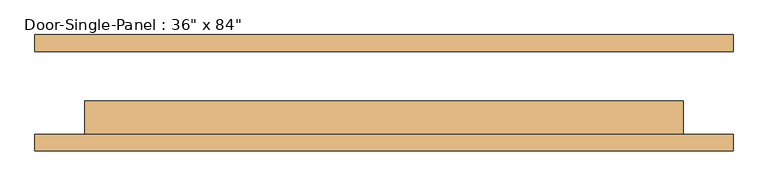
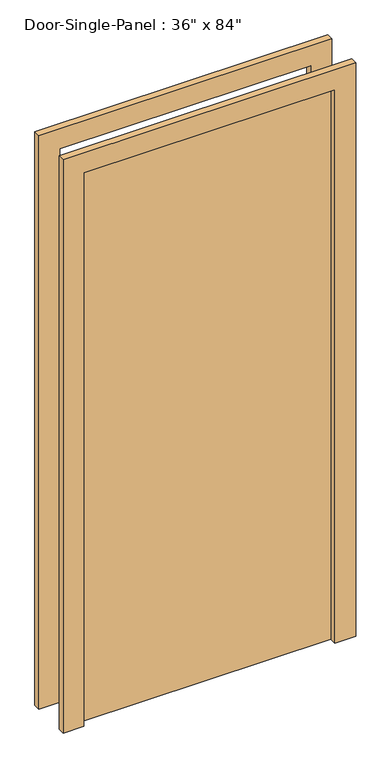
"""IFC4 building model written with IfcOpenShell, lengths in millimetres: door geometry."""

from ifc_helpers import new_model, si_unit, frame, origin, origin_with_axes, place, context, project, spatial, polyline, outline, extrude, source, transform, mapped, element, save


def door_5304b0a0(model_context):
    return source(origin(), model_context, "Body", "SweptSolid", [
        extrude(outline(polyline([(457.2, -12.7), (457.2, -63.5), (-457.2, -63.5), (-457.2, -12.7), (457.2, -12.7)])), origin_with_axes(), (0.0, 0.0, 1.0), 2133.6),
        extrude(outline(polyline([(2209.8, 533.4), (2209.8, -533.4), (0.0, -533.4), (0.0, -457.2), (2133.6, -457.2), (2133.6, 457.2), (0.0, 457.2), (0.0, 533.4), (2209.8, 533.4)])), frame((0.0, 63.5, 0.0), z_axis=(0.0, 1.0, 0.0), x_axis=(0.0, 0.0, 1.0)), (0.0, 0.0, 1.0), 25.4),
        extrude(outline(polyline([(2209.8, -533.4), (0.0, -533.4), (0.0, -457.2), (2133.6, -457.2), (2133.6, 457.2), (0.0, 457.2), (0.0, 533.4), (2209.8, 533.4), (2209.8, -533.4)])), frame((0.0, -88.9, 0.0), z_axis=(0.0, 1.0, 0.0), x_axis=(0.0, 0.0, 1.0)), (0.0, 0.0, 1.0), 25.4),
    ])


if __name__ == "__main__":
    model = new_model("IFC4")
    model_context = context("Model", 3, world=origin())
    ifc_project = project(units=[si_unit("LENGTHUNIT", "METRE", prefix="MILLI")], contexts=[model_context])
    site = spatial("IfcSite", under=ifc_project)
    building = spatial("IfcBuilding", under=site)
    placement = place(None, origin())
    door_shape = door_5304b0a0(model_context)
    element("IfcDoor", 1, ObjectType="Door-Single-Panel : 36\" x 84\"", at=placement, inside=building, context=model_context, shape_type="MappedRepresentation", body=[
        mapped(door_shape, transform((0.0, 0.0, 0.0), x_axis=(1.0, 0.0, 0.0), y_axis=(0.0, 1.0, 0.0), z_axis=(0.0, 0.0, 1.0))),
    ])
    save(model, "model.ifc")

# Revit data of these elements
# Type "Door-Single-Panel : 36\" x 84\""
#   Type Mark = "8"
#   Construction Type Id = "DOOR"
#   Assembly Code = "C1020300"
#   Analytic Construction = "Wooden"
#   Thickness = 0' - 2"
#   Thermal Resistance (R) = 2.5876 (h·ft²·°F)/BTU
#   Swing Angle [instance default] = 90.00°
#   Heat Transfer Coefficient (U) = 0.3865 BTU/(h·ft²·°F)
#   Height = 7' - 0"
#   Trim Projection Ext = 0' - 1"
#   Trim Projection Int = 0' - 1"
#   Trim Width = 0' - 3"
#   Width = 3' - 0"
#   Define Thermal Properties by = 1
#   Panel Material = Wood - Birch - Solid Stained Light Low Gloss
#   Trim Material = Paint - Sienna
#   Visual Light Transmittance = 0
#   Solar Heat Gain Coefficient = 0
#   Function = (empty or 0)
#   Wall Closure = (empty or 0)
# Element 1 (IfcDoor, "Door-Single-Panel : 36\" x 84\"")
#   Materials on its faces: "Paint - Sienna", "Wood - Birch - Solid Stained Light Low Gloss"
# Materials
#   "Wood - Birch - Solid Stained Light Low Gloss": class "Wood", colour RGB 210 159 95, transparency 0, Cost = 0
#   "Paint - Sienna": colour RGB 118 70 51, transparency 0, Cost = 0
